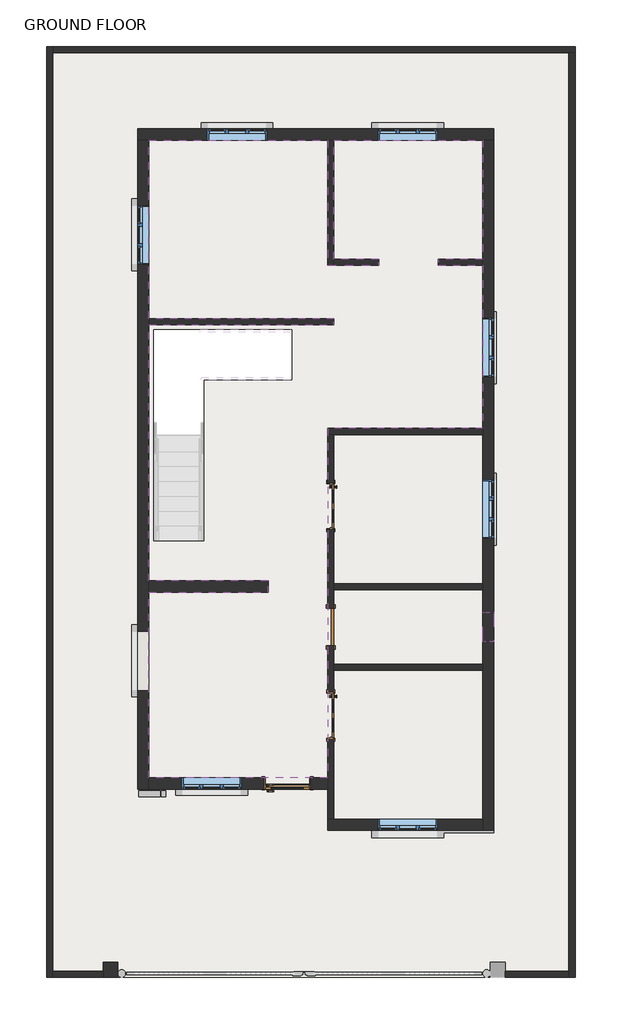
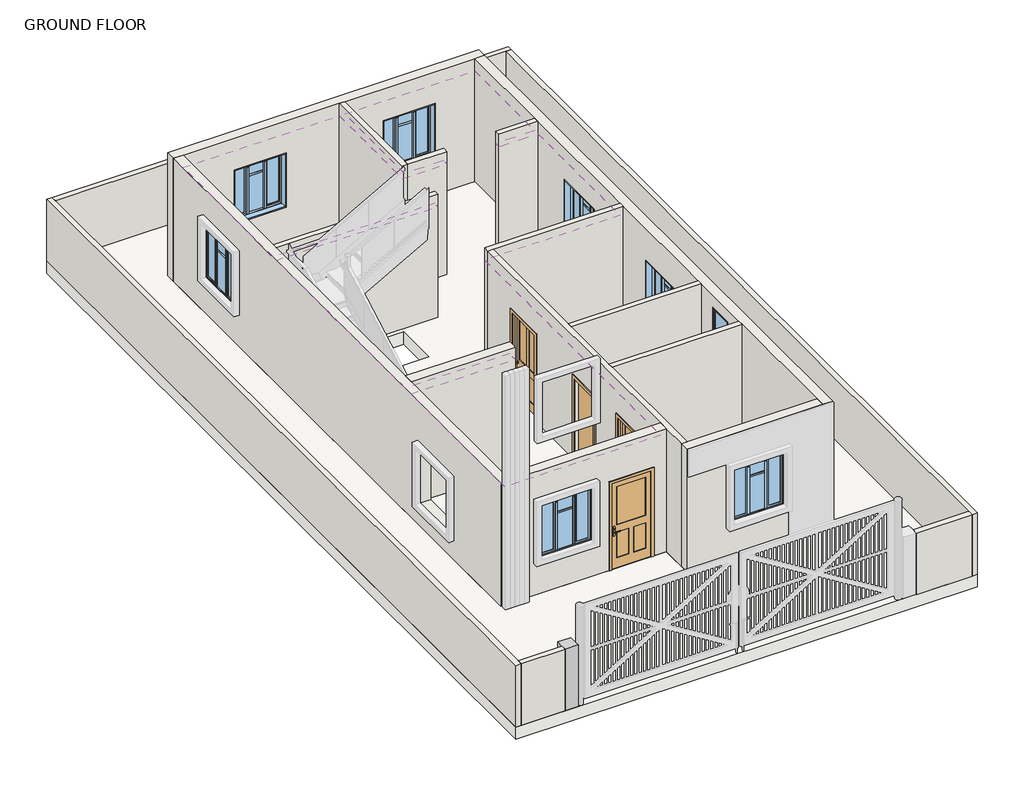
# One storey, part 1 of 4: 19 walls, 8 windows, 4 doors, 3 slabs, 1 column, 1 covering.
"""IFC4 building model written with IfcOpenShell, lengths in millimetres."""

from ifc_helpers import new_model, si_unit, frame, origin, origin_with_axes, place, context, project, spatial, polyline, outline, extrude, faceted_brep, transform, mapped, element, save
from components import door_16625766, door_interior_single_4_panel_wood_interior_common_door_3_x_7_68a706ac, door_e00f436c, window_80340324, window_casement_triple_middle_transom_windows_4_x4_273a115f

model = new_model("IFC4")

# Units and contexts
model_context = context("Model", 3, world=origin())
ifc_project = project(units=[si_unit("LENGTHUNIT", "METRE", prefix="MILLI")], contexts=[model_context])

# Site, building, storey
site = spatial("IfcSite", under=ifc_project)
building = spatial("IfcBuilding", under=site)
storey = spatial("IfcBuildingStorey", under=building, Name="GROUND FLOOR", Elevation=304.8)

# Column
placement = place(None, origin())
element("IfcColumn", 1, ObjectType="Rectangular Column : 1'X 1'", at=placement, inside=storey, context=model_context, shape_type="Brep", body=[
    faceted_brep([(-10104.8610805, -9269.5210084, 304.8), (-10104.8610805, -9574.3210084, 304.8), (-10409.6610805, -9574.3210084, 304.8), (-10409.6610805, -9447.3210084, 304.8), (-10409.6610805, -9269.5210084, 304.8), (-10104.8610805, -9269.5210084, 1828.8), (-10104.8610805, -9574.3210084, 1828.8), (-10409.6610805, -9574.3210084, 1828.8), (-10409.6610805, -9447.3210084, 1828.8), (-10409.6610805, -9269.5210084, 1828.8)], [[[0, 1, 2, 3, 4]], [[5, 6, 1, 0]], [[6, 7, 2, 1]], [[7, 8, 9, 4, 3, 2]], [[9, 5, 0, 4]], [[5, 9, 8, 7, 6]]]),
])

# Covering
element("IfcCovering", 2, ObjectType="2' x 4' ACT System", at=placement, inside=storey, context=model_context, shape_type="SweptSolid", body=[
    extrude(outline(polyline([(-9469.5482439, 3904.0172538), (-9469.5482439, 7561.6172538), (-5810.3607439, 7561.6172538), (-5810.3607439, 4996.2172538), (-4768.9607439, 4996.2172538), (-4768.9607439, 5123.2172538), (-5683.3607439, 5123.2172538), (-5683.3607439, 7561.6172538), (-2635.3607439, 7561.6172538), (-2635.3607439, 5123.2172538), (-3549.7607439, 5123.2172538), (-3549.7607439, 4996.2172538), (-2635.3607439, 4996.2172538), (-2635.3607439, 1659.1157342), (-5810.3607439, 1659.1157342), (-5810.3607439, -5493.9827462), (-9469.5482439, -5493.9827462), (-9469.5482439, -1691.1442658), (-7029.5607439, -1691.1442658), (-7029.5607439, -1462.5442658), (-9469.5482439, -1462.5442658), (-9469.5482439, 3777.0172538), (-5683.3607439, 3777.0172538), (-5683.3607439, 3904.0172538), (-9469.5482439, 3904.0172538)])), frame((0.0, 0.0, 3048.0), z_axis=(0.0, 0.0, 1.0), x_axis=(1.0, 0.0, 0.0)), (0.0, 0.0, 1.0), 57.15),
])

# Doors
door_shape = door_16625766(model_context)
element("IfcDoor", 3, ObjectType="36\" x 84\"", at=placement, inside=storey, context=model_context, shape_type="MappedRepresentation", body=[
    mapped(door_shape, transform((-6635.8607439, -5611.4577462, 304.8), x_axis=(-1.0, 0.0, 0.0), y_axis=(0.0, -1.0, 0.0), z_axis=(0.0, 0.0, 1.0))),
])
door_interior_single_4_panel_wood_interior_common_door_3_x_7_shape = door_interior_single_4_panel_wood_interior_common_door_3_x_7_68a706ac(model_context)
element("IfcDoor", 4, ObjectType="Door-Interior-Single-4_Panel-Wood : INTERIOR COMMON DOOR 3' X 7'", at=placement, inside=storey, context=model_context, shape_type="MappedRepresentation", body=[
    mapped(door_interior_single_4_panel_wood_interior_common_door_3_x_7_shape, transform((-5743.6857439, -4220.9842658, 304.8), x_axis=(0.0, -1.0, 0.0), y_axis=(1.0, 0.0, 0.0), z_axis=(0.0, 0.0, 1.0))),
])
element("IfcDoor", 5, ObjectType="Door-Interior-Single-4_Panel-Wood : INTERIOR COMMON DOOR 3' X 7'", at=placement, inside=storey, context=model_context, shape_type="MappedRepresentation", body=[
    mapped(door_interior_single_4_panel_wood_interior_common_door_3_x_7_shape, transform((-5743.6857439, 66.5357342, 304.8), x_axis=(0.0, -1.0, 0.0), y_axis=(1.0, 0.0, 0.0), z_axis=(0.0, 0.0, 1.0))),
])
door_2_shape = door_e00f436c(model_context)
element("IfcDoor", 6, ObjectType="Single-Flush : 30\" x 80\"", at=placement, inside=storey, context=model_context, shape_type="MappedRepresentation", body=[
    mapped(door_2_shape, transform((-5746.8607439, -2404.8842658, 304.8), x_axis=(0.0, 1.0, 0.0), y_axis=(-1.0, 0.0, 0.0), z_axis=(0.0, 0.0, 1.0))),
])

# Slabs
element("IfcSlab", 7, ObjectType="BATHROOM FLOORING 1'", at=placement, inside=storey, context=model_context, shape_type="SweptSolid", body=[
    extrude(outline(polyline([(-2635.3607439, -1642.8842658), (-2635.3607439, -3166.8842658), (-5683.3607439, -3166.8842658), (-5683.3607439, -1642.8842658), (-2635.3607439, -1642.8842658)])), origin_with_axes(), (0.0, 0.0, 1.0), 304.8),
])
element("IfcSlab", 8, ObjectType="FLOORING GROUND FLOOR 1'", at=placement, inside=storey, context=model_context, shape_type="SweptSolid", body=[
    extrude(outline(polyline([(-2406.7607439, 7790.2172538), (-2406.7607439, -6570.4842658), (-5810.3607439, -6570.4842658), (-5810.3607439, -5722.5827462), (-9698.1482439, -5722.5827462), (-9698.1482439, 7790.2172538), (-2406.7607439, 7790.2172538)]), holes=[polyline([(-2635.3607439, -1642.8842658), (-5683.3607439, -1642.8842658), (-5683.3607439, -3166.8842658), (-2635.3607439, -3166.8842658), (-2635.3607439, -1642.8842658)]), polyline([(-9367.9482439, 3675.4172538), (-9367.9482439, -642.5827462), (-8350.3607439, -642.5827462), (-8350.3607439, 2659.4172538), (-6542.1982439, 2659.4172538), (-6542.1982439, 3675.4172538), (-9367.9482439, 3675.4172538)])]), origin_with_axes(), (0.0, 0.0, 1.0), 304.8),
])
element("IfcSlab", 9, ObjectType="VERANDA FLOORING 1'", at=placement, inside=storey, context=model_context, shape_type="SweptSolid", body=[
    extrude(outline(polyline([(-744.9610805, 9475.6789916), (-744.9610805, -9574.3210084), (-11565.3610805, -9574.3210084), (-11565.3610805, 9475.6789916), (-744.9610805, 9475.6789916)]), holes=[polyline([(-2406.7607439, 7790.2172538), (-9698.1482439, 7790.2172538), (-9698.1482439, -5722.5827462), (-5810.3607439, -5722.5827462), (-5810.3607439, -6570.4842658), (-2406.7607439, -6570.4842658), (-2406.7607439, 7790.2172538)])]), origin_with_axes(), (0.0, 0.0, 1.0), 304.8),
])

# Walls
element("IfcWall", 10, ObjectType="INNER WALL 5\"", at=placement, inside=storey, context=model_context, shape_type="SweptSolid", body=[
    extrude(outline(polyline([(-5683.3607439, 3777.0172538), (-9469.5482439, 3777.0172538), (-9469.5482439, 3904.0172538), (-5683.3607439, 3904.0172538), (-5683.3607439, 3777.0172538)])), frame((0.0, 0.0, 304.8), z_axis=(0.0, 0.0, 1.0), x_axis=(1.0, 0.0, 0.0)), (0.0, 0.0, 1.0), 3048.0),
])
element("IfcWall", 11, ObjectType="INNER WALL 5\"", at=placement, inside=storey, context=model_context, shape_type="Brep", body=[
    faceted_brep([(-2635.3607439, 1659.1157342, 304.8), (-5810.3607439, 1659.1157342, 304.8), (-5810.3607439, 1659.1157342, 3352.8), (-2635.3607439, 1659.1157342, 3352.8), (-2635.3607439, 1532.1157342, 304.8), (-2635.3607439, 1532.1157342, 3352.8), (-5683.3607439, 1532.1157342, 3352.8), (-5810.3607439, 1532.1157342, 3352.8), (-5810.3607439, 1532.1157342, 304.8), (-5683.3607439, 1532.1157342, 304.8)], [[[0, 1, 2, 3]], [[4, 5, 6, 7, 8, 9]], [[1, 0, 4, 9, 8]], [[3, 2, 7, 6, 5]], [[0, 3, 5, 4]], [[2, 1, 8, 7]]]),
])
element("IfcWall", 12, ObjectType="INNER WALL 5\"", at=placement, inside=storey, context=model_context, shape_type="Brep", body=[
    faceted_brep([(-5810.3607439, -416.0642658, 304.8), (-5810.3607439, -2023.8842658, 304.8), (-5810.3607439, -2023.8842658, 2336.8), (-5810.3607439, -2785.8842658, 2336.8), (-5810.3607439, -2785.8842658, 304.8), (-5810.3607439, -3738.3842658, 304.8), (-5810.3607439, -3738.3842658, 2463.8), (-5810.3607439, -4703.5842658, 2463.8), (-5810.3607439, -4703.5842658, 304.8), (-5810.3607439, -5493.9827462, 304.8), (-5810.3607439, -5722.5827462, 304.8), (-5810.3607439, -6341.8842658, 304.8), (-5810.3607439, -6341.8842658, 3352.8), (-5810.3607439, -5722.5827462, 3352.8), (-5810.3607439, -5493.9827462, 3352.8), (-5810.3607439, 1532.1157342, 3352.8), (-5810.3607439, 1532.1157342, 304.8), (-5810.3607439, 549.1357342, 304.8), (-5810.3607439, 549.1357342, 2463.8), (-5810.3607439, -416.0642658, 2463.8), (-5683.3607439, -2023.8842658, 2336.8), (-5683.3607439, -2023.8842658, 304.8), (-5683.3607439, -1642.8842658, 304.8), (-5683.3607439, -1515.8842658, 304.8), (-5683.3607439, -416.0642658, 304.8), (-5683.3607439, -416.0642658, 2463.8), (-5683.3607439, 549.1357342, 2463.8), (-5683.3607439, 549.1357342, 304.8), (-5683.3607439, 1532.1157342, 304.8), (-5683.3607439, 1532.1157342, 3352.8), (-5683.3607439, -1515.8842658, 3352.8), (-5683.3607439, -1642.8842658, 3352.8), (-5683.3607439, -3166.8842658, 3352.8), (-5683.3607439, -3293.8842658, 3352.8), (-5683.3607439, -6341.8842658, 3352.8), (-5683.3607439, -6341.8842658, 304.8), (-5683.3607439, -4703.5842658, 304.8), (-5683.3607439, -4703.5842658, 2463.8), (-5683.3607439, -3738.3842658, 2463.8), (-5683.3607439, -3738.3842658, 304.8), (-5683.3607439, -3293.8842658, 304.8), (-5683.3607439, -3166.8842658, 304.8), (-5683.3607439, -2785.8842658, 304.8), (-5683.3607439, -2785.8842658, 2336.8)], [[[0, 1, 2, 3, 4, 5, 6, 7, 8, 9, 10, 11, 12, 13, 14, 15, 16, 17, 18, 19]], [[20, 21, 22, 23, 24, 25, 26, 27, 28, 29, 30, 31, 32, 33, 34, 35, 36, 37, 38, 39, 40, 41, 42, 43]], [[16, 28, 27, 17]], [[35, 11, 10, 9, 8, 36]], [[42, 41, 40, 39, 5, 4]], [[24, 23, 22, 21, 1, 0]], [[15, 14, 13, 12, 34, 33, 32, 31, 30, 29]], [[16, 15, 29, 28]], [[12, 11, 35, 34]], [[7, 37, 36, 8]], [[37, 7, 6, 38]], [[38, 6, 5, 39]], [[19, 25, 24, 0]], [[25, 19, 18, 26]], [[26, 18, 17, 27]], [[2, 1, 21, 20]], [[3, 2, 20, 43]], [[4, 3, 43, 42]]]),
])
element("IfcWall", 13, ObjectType="INNER WALL 5\"", at=placement, inside=storey, context=model_context, shape_type="SweptSolid", body=[
    extrude(outline(polyline([(-2635.3607439, -3293.8842658), (-5683.3607439, -3293.8842658), (-5683.3607439, -3166.8842658), (-2635.3607439, -3166.8842658), (-2635.3607439, -3293.8842658)])), frame((0.0, 0.0, 304.8), z_axis=(0.0, 0.0, 1.0), x_axis=(1.0, 0.0, 0.0)), (0.0, 0.0, 1.0), 3048.0),
])
element("IfcWall", 14, ObjectType="INNER WALL 5\"", at=placement, inside=storey, context=model_context, shape_type="SweptSolid", body=[
    extrude(outline(polyline([(-2635.3607439, -1642.8842658), (-5683.3607439, -1642.8842658), (-5683.3607439, -1515.8842658), (-2635.3607439, -1515.8842658), (-2635.3607439, -1642.8842658)])), frame((0.0, 0.0, 304.8), z_axis=(0.0, 0.0, 1.0), x_axis=(1.0, 0.0, 0.0)), (0.0, 0.0, 1.0), 3048.0),
])
element("IfcWall", 15, ObjectType="INNER WALL 5\"", at=placement, inside=storey, context=model_context, shape_type="Brep", body=[
    faceted_brep([(-5810.3607439, 7561.6172538, 304.8), (-5810.3607439, 4996.2172538, 304.8), (-5810.3607439, 4996.2172538, 3352.8), (-5810.3607439, 7561.6172538, 3352.8), (-5683.3607439, 7561.6172538, 304.8), (-5683.3607439, 7561.6172538, 3352.8), (-5683.3607439, 5123.2172538, 3352.8), (-5683.3607439, 4996.2172538, 3352.8), (-5683.3607439, 4996.2172538, 304.8), (-5683.3607439, 5123.2172538, 304.8)], [[[0, 1, 2, 3]], [[4, 5, 6, 7, 8, 9]], [[1, 0, 4, 9, 8]], [[3, 2, 7, 6, 5]], [[0, 3, 5, 4]], [[2, 1, 8, 7]]]),
])
element("IfcWall", 16, ObjectType="INNER WALL 5\"", at=placement, inside=storey, context=model_context, shape_type="SweptSolid", body=[
    extrude(outline(polyline([(-4768.9607439, 4996.2172538), (-5683.3607439, 4996.2172538), (-5683.3607439, 5123.2172538), (-4768.9607439, 5123.2172538), (-4768.9607439, 4996.2172538)])), frame((0.0, 0.0, 304.8), z_axis=(0.0, 0.0, 1.0), x_axis=(1.0, 0.0, 0.0)), (0.0, 0.0, 1.0), 3048.0),
])
element("IfcWall", 17, ObjectType="INNER WALL 5\"", at=placement, inside=storey, context=model_context, shape_type="SweptSolid", body=[
    extrude(outline(polyline([(-2635.3607439, 4996.2172538), (-3549.7607439, 4996.2172538), (-3549.7607439, 5123.2172538), (-2635.3607439, 5123.2172538), (-2635.3607439, 4996.2172538)])), frame((0.0, 0.0, 304.8), z_axis=(0.0, 0.0, 1.0), x_axis=(1.0, 0.0, 0.0)), (0.0, 0.0, 1.0), 3048.0),
])
element("IfcWall", 18, ObjectType="INNER WALL 5\"", at=placement, inside=storey, context=model_context, shape_type="Brep", body=[
    faceted_brep([(-11565.3610805, 9475.6789916, 304.8), (-11565.3610805, -9574.3210084, 304.8), (-11565.3610805, -9574.3210084, 1828.8), (-11565.3610805, 9475.6789916, 1828.8), (-11438.3610805, 9475.6789916, 304.8), (-11438.3610805, 9475.6789916, 1828.8), (-11438.3610805, 9348.6789916, 1828.8), (-11438.3610805, -9447.3210084, 1828.8), (-11438.3610805, -9574.3210084, 1828.8), (-11438.3610805, -9574.3210084, 304.8), (-11438.3610805, -9447.3210084, 304.8), (-11438.3610805, 9348.6789916, 304.8)], [[[0, 1, 2, 3]], [[4, 5, 6, 7, 8, 9, 10, 11]], [[1, 0, 4, 11, 10, 9]], [[3, 2, 8, 7, 6, 5]], [[0, 3, 5, 4]], [[2, 1, 9, 8]]]),
])
element("IfcWall", 19, ObjectType="INNER WALL 5\"", at=placement, inside=storey, context=model_context, shape_type="Brep", body=[
    faceted_brep([(-11438.3610805, 9348.6789916, 304.8), (-871.9610805, 9348.6789916, 304.8), (-744.9610805, 9348.6789916, 304.8), (-744.9610805, 9348.6789916, 1828.8), (-871.9610805, 9348.6789916, 1828.8), (-11438.3610805, 9348.6789916, 1828.8), (-11438.3610805, 9475.6789916, 304.8), (-11438.3610805, 9475.6789916, 1828.8), (-744.9610805, 9475.6789916, 1828.8), (-744.9610805, 9475.6789916, 304.8)], [[[0, 1, 2, 3, 4, 5]], [[6, 7, 8, 9]], [[2, 1, 0, 6, 9]], [[5, 4, 3, 8, 7]], [[0, 5, 7, 6]], [[3, 2, 9, 8]]]),
])
element("IfcWall", 20, ObjectType="INNER WALL 5\"", at=placement, inside=storey, context=model_context, shape_type="Brep", body=[
    faceted_brep([(-871.9610805, 9348.6789916, 304.8), (-871.9610805, -9447.3210084, 304.8), (-871.9610805, -9574.3210084, 304.8), (-871.9610805, -9574.3210084, 1828.8), (-871.9610805, -9447.3210084, 1828.8), (-871.9610805, 9348.6789916, 1828.8), (-744.9610805, 9348.6789916, 304.8), (-744.9610805, 9348.6789916, 1828.8), (-744.9610805, -9574.3210084, 1828.8), (-744.9610805, -9574.3210084, 304.8)], [[[0, 1, 2, 3, 4, 5]], [[6, 7, 8, 9]], [[2, 1, 0, 6, 9]], [[5, 4, 3, 8, 7]], [[0, 5, 7, 6]], [[3, 2, 9, 8]]]),
])
element("IfcWall", 21, ObjectType="INNER WALL 5\"", at=placement, inside=storey, context=model_context, shape_type="SweptSolid", body=[
    extrude(outline(polyline([(-2180.0610805, -9447.3210084), (-871.9610805, -9447.3210084), (-871.9610805, -9574.3210084), (-2180.0610805, -9574.3210084), (-2180.0610805, -9447.3210084)])), frame((0.0, 0.0, 304.8), z_axis=(0.0, 0.0, 1.0), x_axis=(1.0, 0.0, 0.0)), (0.0, 0.0, 1.0), 1524.0),
])
element("IfcWall", 22, ObjectType="INNER WALL 5\"", at=placement, inside=storey, context=model_context, shape_type="SweptSolid", body=[
    extrude(outline(polyline([(-10409.6610805, -9574.3210084), (-11438.3610805, -9574.3210084), (-11438.3610805, -9447.3210084), (-10409.6610805, -9447.3210084), (-10409.6610805, -9574.3210084)])), frame((0.0, 0.0, 304.8), z_axis=(0.0, 0.0, 1.0), x_axis=(1.0, 0.0, 0.0)), (0.0, 0.0, 1.0), 1524.0),
])
element("IfcWall", 23, ObjectType="WALL 9\"", at=placement, inside=storey, context=model_context, shape_type="Brep", body=[
    faceted_brep([(-9698.1482439, 7561.6172538, 304.8), (-9469.5482439, 7561.6172538, 304.8), (-5810.3607439, 7561.6172538, 304.8), (-5683.3607439, 7561.6172538, 304.8), (-2635.3607439, 7561.6172538, 304.8), (-2406.7607439, 7561.6172538, 304.8), (-2406.7607439, 7561.6172538, 3352.8), (-2635.3607439, 7561.6172538, 3352.8), (-5683.3607439, 7561.6172538, 3352.8), (-5810.3607439, 7561.6172538, 3352.8), (-9469.5482439, 7561.6172538, 3352.8), (-9698.1482439, 7561.6172538, 3352.8), (-7055.7544939, 7561.6172538, 2565.4), (-7055.7544939, 7561.6172538, 1219.2), (-8274.9544939, 7561.6172538, 1219.2), (-8274.9544939, 7561.6172538, 2565.4), (-3562.4607439, 7561.6172538, 2565.4), (-3562.4607439, 7561.6172538, 1219.2), (-4781.6607439, 7561.6172538, 1219.2), (-4781.6607439, 7561.6172538, 2565.4), (-9698.1482439, 7790.2172538, 304.8), (-9698.1482439, 7790.2172538, 3352.8), (-2406.7607439, 7790.2172538, 3352.8), (-2406.7607439, 7790.2172538, 304.8), (-7055.7544939, 7790.2172538, 2565.4), (-8274.9544939, 7790.2172538, 2565.4), (-8274.9544939, 7790.2172538, 1219.2), (-7055.7544939, 7790.2172538, 1219.2), (-3562.4607439, 7790.2172538, 2565.4), (-4781.6607439, 7790.2172538, 2565.4), (-4781.6607439, 7790.2172538, 1219.2), (-3562.4607439, 7790.2172538, 1219.2)], [[[0, 1, 2, 3, 4, 5, 6, 7, 8, 9, 10, 11], [12, 13, 14, 15], [16, 17, 18, 19]], [[20, 21, 22, 23], [24, 25, 26, 27], [28, 29, 30, 31]], [[5, 4, 3, 2, 1, 0, 20, 23]], [[11, 10, 9, 8, 7, 6, 22, 21]], [[6, 5, 23, 22]], [[0, 11, 21, 20]], [[13, 12, 24, 27]], [[14, 13, 27, 26]], [[15, 14, 26, 25]], [[12, 15, 25, 24]], [[17, 16, 28, 31]], [[18, 17, 31, 30]], [[19, 18, 30, 29]], [[16, 19, 29, 28]]]),
])
element("IfcWall", 24, ObjectType="WALL 9\"", at=placement, inside=storey, context=model_context, shape_type="Brep", body=[
    faceted_brep([(-2635.3607439, 7561.6172538, 304.8), (-2635.3607439, 5123.2172538, 304.8), (-2635.3607439, 4996.2172538, 304.8), (-2635.3607439, 1659.1157342, 304.8), (-2635.3607439, 1532.1157342, 304.8), (-2635.3607439, -1515.8842658, 304.8), (-2635.3607439, -1642.8842658, 304.8), (-2635.3607439, -3166.8842658, 304.8), (-2635.3607439, -3293.8842658, 304.8), (-2635.3607439, -6341.8842658, 304.8), (-2635.3607439, -6570.4842658, 304.8), (-2635.3607439, -6570.4842658, 3352.8), (-2635.3607439, -6341.8842658, 3352.8), (-2635.3607439, -3293.8842658, 3352.8), (-2635.3607439, -3166.8842658, 3352.8), (-2635.3607439, -1642.8842658, 3352.8), (-2635.3607439, -1515.8842658, 3352.8), (-2635.3607439, 1532.1157342, 3352.8), (-2635.3607439, 1659.1157342, 3352.8), (-2635.3607439, 4996.2172538, 3352.8), (-2635.3607439, 5123.2172538, 3352.8), (-2635.3607439, 7561.6172538, 3352.8), (-2635.3607439, 2705.366494, 2565.4), (-2635.3607439, 2705.366494, 1219.2), (-2635.3607439, 3924.566494, 1219.2), (-2635.3607439, 3924.566494, 2565.4), (-2635.3607439, -601.4842658, 2565.4), (-2635.3607439, -601.4842658, 1219.2), (-2635.3607439, 617.7157342, 1219.2), (-2635.3607439, 617.7157342, 2565.4), (-2635.3607439, -2100.0842658, 3048.0), (-2635.3607439, -2709.6842658, 3048.0), (-2635.3607439, -2709.6842658, 2438.4), (-2635.3607439, -2100.0842658, 2438.4), (-2406.7607439, 7561.6172538, 304.8), (-2406.7607439, 7561.6172538, 3352.8), (-2406.7607439, -6570.4842658, 3352.8), (-2406.7607439, -6570.4842658, 304.8), (-2406.7607439, 2705.366494, 2565.4), (-2406.7607439, 3924.566494, 2565.4), (-2406.7607439, 3924.566494, 1219.2), (-2406.7607439, 2705.366494, 1219.2), (-2406.7607439, -601.4842658, 2565.4), (-2406.7607439, 617.7157342, 2565.4), (-2406.7607439, 617.7157342, 1219.2), (-2406.7607439, -601.4842658, 1219.2), (-2406.7607439, -2100.0842658, 3048.0), (-2406.7607439, -2100.0842658, 2438.4), (-2406.7607439, -2709.6842658, 2438.4), (-2406.7607439, -2709.6842658, 3048.0)], [[[0, 1, 2, 3, 4, 5, 6, 7, 8, 9, 10, 11, 12, 13, 14, 15, 16, 17, 18, 19, 20, 21], [22, 23, 24, 25], [26, 27, 28, 29], [30, 31, 32, 33]], [[34, 35, 36, 37], [38, 39, 40, 41], [42, 43, 44, 45], [46, 47, 48, 49]], [[10, 9, 8, 7, 6, 5, 4, 3, 2, 1, 0, 34, 37]], [[21, 20, 19, 18, 17, 16, 15, 14, 13, 12, 11, 36, 35]], [[0, 21, 35, 34]], [[11, 10, 37, 36]], [[23, 22, 38, 41]], [[24, 23, 41, 40]], [[25, 24, 40, 39]], [[22, 25, 39, 38]], [[27, 26, 42, 45]], [[28, 27, 45, 44]], [[29, 28, 44, 43]], [[26, 29, 43, 42]], [[47, 46, 30, 33]], [[48, 47, 33, 32]], [[49, 48, 32, 31]], [[46, 49, 31, 30]]]),
])
element("IfcWall", 25, ObjectType="WALL 9\"", at=placement, inside=storey, context=model_context, shape_type="Brep", body=[
    faceted_brep([(-2635.3607439, -6341.8842658, 304.8), (-5683.3607439, -6341.8842658, 304.8), (-5810.3607439, -6341.8842658, 304.8), (-5810.3607439, -6341.8842658, 3352.8), (-5683.3607439, -6341.8842658, 3352.8), (-2635.3607439, -6341.8842658, 3352.8), (-4781.6607439, -6341.8842658, 2565.4), (-4781.6607439, -6341.8842658, 1219.2), (-3562.4607439, -6341.8842658, 1219.2), (-3562.4607439, -6341.8842658, 2565.4), (-2635.3607439, -6570.4842658, 304.8), (-2635.3607439, -6570.4842658, 3352.8), (-5810.3607439, -6570.4842658, 3352.8), (-5810.3607439, -6570.4842658, 304.8), (-4781.6607439, -6570.4842658, 2565.4), (-3562.4607439, -6570.4842658, 2565.4), (-3562.4607439, -6570.4842658, 1219.2), (-4781.6607439, -6570.4842658, 1219.2)], [[[0, 1, 2, 3, 4, 5], [6, 7, 8, 9]], [[10, 11, 12, 13], [14, 15, 16, 17]], [[2, 1, 0, 10, 13]], [[5, 4, 3, 12, 11]], [[0, 5, 11, 10]], [[3, 2, 13, 12]], [[7, 6, 14, 17]], [[8, 7, 17, 16]], [[9, 8, 16, 15]], [[6, 9, 15, 14]]]),
])
element("IfcWall", 26, ObjectType="WALL 9\"", at=placement, inside=storey, context=model_context, shape_type="Brep", body=[
    faceted_brep([(-9698.1482439, 7561.6172538, 304.8), (-9698.1482439, -5722.5827462, 304.8), (-9698.1482439, -5722.5827462, 3352.8), (-9698.1482439, 7561.6172538, 3352.8), (-9698.1482439, 6228.1172538, 2565.4), (-9698.1482439, 5008.9172538, 2565.4), (-9698.1482439, 5008.9172538, 1219.2), (-9698.1482439, 6228.1172538, 1219.2), (-9698.1482439, -2491.2442658, 2260.6), (-9698.1482439, -3710.4442658, 2260.6), (-9698.1482439, -3710.4442658, 914.4), (-9698.1482439, -2491.2442658, 914.4), (-9469.5482439, 7561.6172538, 304.8), (-9469.5482439, 7561.6172538, 3352.8), (-9469.5482439, 3904.0172538, 3352.8), (-9469.5482439, 3777.0172538, 3352.8), (-9469.5482439, -1462.5442658, 3352.8), (-9469.5482439, -1691.1442658, 3352.8), (-9469.5482439, -5493.9827462, 3352.8), (-9469.5482439, -5722.5827462, 3352.8), (-9469.5482439, -5722.5827462, 304.8), (-9469.5482439, -5493.9827462, 304.8), (-9469.5482439, -1691.1442658, 304.8), (-9469.5482439, -1462.5442658, 304.8), (-9469.5482439, 3777.0172538, 304.8), (-9469.5482439, 3904.0172538, 304.8), (-9469.5482439, 6228.1172538, 2565.4), (-9469.5482439, 6228.1172538, 1219.2), (-9469.5482439, 5008.9172538, 1219.2), (-9469.5482439, 5008.9172538, 2565.4), (-9469.5482439, -2491.2442658, 2260.6), (-9469.5482439, -2491.2442658, 914.4), (-9469.5482439, -3710.4442658, 914.4), (-9469.5482439, -3710.4442658, 2260.6)], [[[0, 1, 2, 3], [4, 5, 6, 7], [8, 9, 10, 11]], [[12, 13, 14, 15, 16, 17, 18, 19, 20, 21, 22, 23, 24, 25], [26, 27, 28, 29], [30, 31, 32, 33]], [[1, 0, 12, 25, 24, 23, 22, 21, 20]], [[3, 2, 19, 18, 17, 16, 15, 14, 13]], [[0, 3, 13, 12]], [[2, 1, 20, 19]], [[27, 26, 4, 7]], [[28, 27, 7, 6]], [[29, 28, 6, 5]], [[26, 29, 5, 4]], [[31, 30, 8, 11]], [[32, 31, 11, 10]], [[33, 32, 10, 9]], [[30, 33, 9, 8]]]),
])
element("IfcWall", 27, ObjectType="WALL 9\"", at=placement, inside=storey, context=model_context, shape_type="SweptSolid", body=[
    extrude(outline(polyline([(3352.8, -5810.3607439), (3352.8, -9469.5482439), (304.8, -9469.5482439), (304.8, -7118.4607439), (2463.8, -7118.4607439), (2463.8, -6153.2607439), (304.8, -6153.2607439), (304.8, -5810.3607439), (3352.8, -5810.3607439)]), holes=[polyline([(2565.4, -8796.4482439), (2565.4, -7577.2482439), (1219.2, -7577.2482439), (1219.2, -8796.4482439), (2565.4, -8796.4482439)])]), frame((0.0, -5722.5827462, 0.0), z_axis=(0.0, 1.0, 0.0), x_axis=(0.0, 0.0, 1.0)), (0.0, 0.0, 1.0), 228.6),
])
element("IfcWall", 28, ObjectType="WALL 9\"", at=placement, inside=storey, context=model_context, shape_type="SweptSolid", body=[
    extrude(outline(polyline([(-7029.5607439, -1691.1442658), (-9469.5482439, -1691.1442658), (-9469.5482439, -1462.5442658), (-7029.5607439, -1462.5442658), (-7029.5607439, -1691.1442658)])), frame((0.0, 0.0, 304.8), z_axis=(0.0, 0.0, 1.0), x_axis=(1.0, 0.0, 0.0)), (0.0, 0.0, 1.0), 3048.0),
])

# Windows
window_shape = window_80340324(model_context)
element("IfcWindow", 29, ObjectType="Fixed : 24\" x 24\"", at=placement, inside=storey, context=model_context, shape_type="MappedRepresentation", body=[
    mapped(window_shape, transform((-2521.0607439, -2366.7842658, 1524.0), x_axis=(0.0, 1.0, 0.0), y_axis=(-1.0, 0.0, 0.0), z_axis=(0.0, 0.0, 1.0))),
])
window_casement_triple_middle_transom_windows_4_x4_shape = window_casement_triple_middle_transom_windows_4_x4_273a115f(model_context)
element("IfcWindow", 30, ObjectType="Window-Casement-Triple-Middle-Transom : WINDOWS 4'X4'", at=placement, inside=storey, context=model_context, shape_type="MappedRepresentation", body=[
    mapped(window_casement_triple_middle_transom_windows_4_x4_shape, transform((-7665.3544939, 7675.9172538, 304.8), x_axis=(1.0, 0.0, 0.0), y_axis=(0.0, 1.0, 0.0), z_axis=(0.0, 0.0, 1.0))),
])
element("IfcWindow", 31, ObjectType="Window-Casement-Triple-Middle-Transom : WINDOWS 4'X4'", at=placement, inside=storey, context=model_context, shape_type="MappedRepresentation", body=[
    mapped(window_casement_triple_middle_transom_windows_4_x4_shape, transform((-4172.0607439, 7675.9172538, 304.8), x_axis=(1.0, 0.0, 0.0), y_axis=(0.0, 1.0, 0.0), z_axis=(0.0, 0.0, 1.0))),
])
element("IfcWindow", 32, ObjectType="Window-Casement-Triple-Middle-Transom : WINDOWS 4'X4'", at=placement, inside=storey, context=model_context, shape_type="MappedRepresentation", body=[
    mapped(window_casement_triple_middle_transom_windows_4_x4_shape, transform((-2521.0607439, 3314.966494, 304.8), x_axis=(0.0, -1.0, 0.0), y_axis=(1.0, 0.0, 0.0), z_axis=(0.0, 0.0, 1.0))),
])
element("IfcWindow", 33, ObjectType="Window-Casement-Triple-Middle-Transom : WINDOWS 4'X4'", at=placement, inside=storey, context=model_context, shape_type="MappedRepresentation", body=[
    mapped(window_casement_triple_middle_transom_windows_4_x4_shape, transform((-2521.0607439, 8.1157342, 304.8), x_axis=(0.0, -1.0, 0.0), y_axis=(1.0, 0.0, 0.0), z_axis=(0.0, 0.0, 1.0))),
])
element("IfcWindow", 34, ObjectType="Window-Casement-Triple-Middle-Transom : WINDOWS 4'X4'", at=placement, inside=storey, context=model_context, shape_type="MappedRepresentation", body=[
    mapped(window_casement_triple_middle_transom_windows_4_x4_shape, transform((-4172.0607439, -6456.1842658, 304.8), x_axis=(-1.0, 0.0, 0.0), y_axis=(0.0, -1.0, 0.0), z_axis=(0.0, 0.0, 1.0))),
])
element("IfcWindow", 35, ObjectType="Window-Casement-Triple-Middle-Transom : WINDOWS 4'X4'", at=placement, inside=storey, context=model_context, shape_type="MappedRepresentation", body=[
    mapped(window_casement_triple_middle_transom_windows_4_x4_shape, transform((-8186.8482439, -5608.2827462, 304.8), x_axis=(-1.0, 0.0, 0.0), y_axis=(0.0, -1.0, 0.0), z_axis=(0.0, 0.0, 1.0))),
])
element("IfcWindow", 36, ObjectType="Window-Casement-Triple-Middle-Transom : WINDOWS 4'X4'", at=placement, inside=storey, context=model_context, shape_type="MappedRepresentation", body=[
    mapped(window_casement_triple_middle_transom_windows_4_x4_shape, transform((-9583.8482439, 5618.5172538, 304.8), x_axis=(0.0, 1.0, 0.0), y_axis=(-1.0, 0.0, 0.0), z_axis=(0.0, 0.0, 1.0))),
])

save(model, "model.ifc")

# Revit data of these elements
# Type "Rectangular Column : 1'X 1'"
#   Assembly Code = "B1010200"
#   Depth = 1' - 0"
#   Offset Base = 0' - 0"
#   Offset Top = 0' - 0"
#   Width = 1' - 0"
# Type "2' x 4' ACT System"
#   Assembly Code = "C3030210"
#   built-in parameter 1002203 = 1 (stored number, unit not read)
#   built-in parameter 1002202 = 1 (stored number, unit not read)
#   Layers, outside or top first: 0' - 1 5/8" "Default" (function 1); 0' - 0 5/8" "Acoustic Ceiling Tile 24 x 48" (function 5)
# Type "36\" x 84\""
#   Type Mark = "8"
#   Assembly Code = "B2030100"
#   Analytic Construction = "French door, wood frame with single glass"
#   Top Rail = 0' - 4 3/4"
#   Threshold Offset [instance default] = 0' - 0 1/2"
#   Thickness = 0' - 1 3/8"
#   Thermal Resistance (R) = 1.0696 (h·ft²·°F)/BTU
#   Swing Angle [instance default] = 90.00°
#   Stiles = 0' - 4 3/4"
#   Rough Width = 3' - 2"
#   Rough Height = 7' - 1"
#   Lock Rail = 0' - 7 1/8"
#   Height = 7' - 0"
#   Width = 3' - 0"
#   Heat Transfer Coefficient (U) = 0.9350 BTU/(h·ft²·°F)
#   Door Offset [instance default] = 0' - 0"
#   Bottom Rail = 0' - 9 1/2"
#   Threshold [instance default] = yes
#   Function = 1
#   Exterior Trim [instance default] = yes
#   Trim Material = Cherry
#   Threshold Material = Cherry
#   Panel Material = Cherry
#   Glazing = Glass
#   Frame Material = Cherry
#   Door Handle Material = Aluminum
#   Visual Light Transmittance = 0
#   Solar Heat Gain Coefficient = 0
#   Wall Closure = (empty or 0)
#   Construction Type = (empty or 0)
# Type "Door-Interior-Single-4_Panel-Wood : INTERIOR COMMON DOOR 3' X 7'"
#   Type Mark = "11"
#   Assembly Code = "C1020300"
#   Analytic Construction = "Wooden"
#   Top Rail = 0' - 4 11/16"
#   Thickness = 0' - 1 3/8"
#   Thermal Resistance (R) = 2.5876 (h·ft²·°F)/BTU
#   Swing Angle [instance default] = 90.00°
#   Stiles = 0' - 4 3/4"
#   Rough Width = 3' - 2"
#   Rough Height = 7' - 1"
#   Mullion = 0' - 4 1/2"
#   Lock Rail = 0' - 7 1/2"
#   Height = 7' - 0"
#   Width = 3' - 0"
#   Heat Transfer Coefficient (U) = 0.3865 BTU/(h·ft²·°F)
#   Bottom Rail = 0' - 9 1/8"
#   Trim Material = Cherry
#   Panel Material = Cherry
#   Frame Material = Cherry
#   Door Handle Material = Aluminum
#   Visual Light Transmittance = 0
#   Solar Heat Gain Coefficient = 0
#   Wall Closure = (empty or 0)
#   Function = (empty or 0)
# Type "Single-Flush : 30\" x 80\""
#   Type Mark = "5"
#   Construction Type Id = "MDOOR"
#   Assembly Code = "C1020"
#   Analytic Construction = "Metal"
#   Thickness = 0' - 2"
#   Heat Transfer Coefficient (U) = 0.651978 BTU/(h·ft²·°F)
#   Height = 6' - 8"
#   Trim Projection Ext = 0' - 1"
#   Trim Projection Int = 0' - 1"
#   Trim Width = 0' - 3"
#   Width = 2' - 6"
#   Define Thermal Properties by = 1
#   Define Thermal Properties by = 1
#   Door Material = Door - Panel
#   Frame Material = Door - Frame
#   Visual Light Transmittance = 0
#   Solar Heat Gain Coefficient = 0
#   Function = (empty or 0)
#   Wall Closure = (empty or 0)
# Type "BATHROOM FLOORING 1'"
#   Assembly Code = "B1010"
#   Function = 0
#   Layers, outside or top first: 1' - 0" "BATHROOM FLOORING" (function 1)
# Type "FLOORING GROUND FLOOR 1'"
#   Assembly Code = "B1010"
#   Function = 0
#   Layers, outside or top first: 1' - 0" "MARBLE FLOORING 1'" (function 1)
# Type "VERANDA FLOORING 1'"
#   Assembly Code = "B1010"
#   Function = 0
#   Layers, outside or top first: 1' - 0" "VERANDA FLOORING" (function 1)
# Type "INNER WALL 5\""
#   Assembly Code = "B2010"
# Type "WALL 9\""
#   Assembly Code = "B2010"
# Type "Fixed : 24\" x 24\""
#   Type Mark = "3"
#   Construction Type Id = "GSP4R"
#   Assembly Code = "B2020100"
#   Analytic Construction = "1/8 in Pilkington single glazing"
#   Visual Light Transmittance = 0.9
#   Solar Heat Gain Coefficient = 0.78
#   Heat Transfer Coefficient (U) = 0.6496 BTU/(h·ft²·°F)
#   Height = 2' - 0"
#   Default Sill Height = 3' - 0"
#   Width = 2' - 0"
#   Window Inset = 0' - 0 3/4"
#   Define Thermal Properties by = 1
#   Define Thermal Properties by = 1
#   Glass Pane Material = Glass
#   Sash Material = Sash
#   Wall Closure = (empty or 0)
# Type "Window-Casement-Triple-Middle-Transom : WINDOWS 4'X4'"
#   Type Mark = "21"
#   Fire Rating = "0.5h"
#   Assembly Code = "B2020100"
#   Analytic Construction = "Double glazing - domestic"
#   Window Width = 1' - 4"
#   Window Inset [instance default] = 0' - 0 5/8"
#   Wall Thickness [instance default] = 0' - 6"
#   Visual Light Transmittance = 0.81
#   Transom Height Ratio = 0.3
#   Thermal Resistance (R) = 1.8146 (h·ft²·°F)/BTU
#   Solar Heat Gain Coefficient = 0.76
#   Rough Width = 4' - 0 1/2"
#   Rough Height = 4' - 5 1/2"
#   Heat Transfer Coefficient (U) = 0.5511 BTU/(h·ft²·°F)
#   Height = 4' - 5"
#   Transom Height = 1' - 3.9"
#   Frame Gap 3 [instance default] = 0' - 1 83/128"
#   Frame Gap 2 [instance default] = 0' - 0 5/8"
#   Frame Gap 1 = 0' - 1 51/128"
#   Default Sill Height = 3' - 0"
#   Width = 4' - 0"
#   Frame Material = Metal - Aluminum
#   Glass Panel Material = Glass
#   Wall Closure = (empty or 0)
# Element 1 (IfcColumn, "Rectangular Column : 1'X 1'")
#   Phase Created = New Construction
# Element 2 (IfcCovering, "2' x 4' ACT System")
#   Height Offset From Level = 9' - 0"
#   Phase Created = New Construction
#   Materials on its faces: "Acoustic Ceiling Tile 24 x 48", "Default"
# Element 3 (IfcDoor, "36\" x 84\"")
#   Threshold Offset = 0' - 0 1/2"
#   Swing Angle = 90.00°
#   Door Offset = 0' - 0"
#   Threshold = yes
#   Exterior Trim = yes
#   Phase Created = New Construction
#   Materials on its faces: "Cherry", "Aluminum", "Glass"
# Elements 4, 5 (IfcDoor, "Door-Interior-Single-4_Panel-Wood : INTERIOR COMMON DOOR 3' X 7'")
#   Swing Angle = 90.00°
#   Phase Created = New Construction
#   Materials on its faces: "Cherry", "Aluminum"
# Element 6 (IfcDoor, "Single-Flush : 30\" x 80\"")
#   Phase Created = New Construction
#   Materials on its faces: "Door - Frame", "Door - Panel"
# Element 7 (IfcSlab, "BATHROOM FLOORING 1'")
#   Height Offset From Level = 0' - 0"
#   Phase Created = New Construction
#   Materials on its faces: "BATHROOM FLOORING"
# Element 8 (IfcSlab, "FLOORING GROUND FLOOR 1'")
#   Height Offset From Level = 0' - 0"
#   Phase Created = New Construction
#   Materials on its faces: "MARBLE FLOORING 1'"
# Element 9 (IfcSlab, "VERANDA FLOORING 1'")
#   Height Offset From Level = 0' - 0"
#   Phase Created = New Construction
#   Materials on its faces: "VERANDA FLOORING"
# Elements 10, 11, 12, 13, 14, 15, 16, 17 (IfcWall, "INNER WALL 5\"")
#   Top Offset = 0' - 0"
#   Base Offset = 0' - 0"
#   wall height = 10' - 0"
#   Phase Created = New Construction
#   Base Constraint = GROUND FLOOR
#   Top Constraint = Level 2
#   Materials on its faces: "SAGE GREEN"
# Elements 18, 19, 20, 21, 22 (IfcWall, "INNER WALL 5\"")
#   Top Offset = 0' - 0"
#   Base Offset = 0' - 0"
#   Unconnected Height = 5' - 0"
#   wall height = 5' - 0"
#   Phase Created = New Construction
#   Base Constraint = GROUND FLOOR
# Elements 23, 24, 25, 26, 27, 28 (IfcWall, "WALL 9\"")
#   Top Offset = 0' - 0"
#   Base Offset = 0' - 0"
#   wall height = 10' - 0"
#   Phase Created = New Construction
#   Base Constraint = GROUND FLOOR
#   Top Constraint = Level 2
#   Materials on its faces: "SAGE GREEN"
# Element 29 (IfcWindow, "Fixed : 24\" x 24\"")
#   Mark = "12"
#   Phase Created = New Construction
#   Materials on its faces: "Sash", "Glass"
# Element 30 (IfcWindow, "Window-Casement-Triple-Middle-Transom : WINDOWS 4'X4'")
#   Mark = "5"
#   Window Inset = 0' - 0 5/8"
#   Frame Gap 3 = 0' - 1 83/128"
#   Frame Gap 2 = 0' - 0 5/8"
#   Phase Created = New Construction
#   Materials on its faces: "Metal - Aluminum", "Glass"
# Element 31 (IfcWindow, "Window-Casement-Triple-Middle-Transom : WINDOWS 4'X4'")
#   Mark = "6"
#   Window Inset = 0' - 0 5/8"
#   Frame Gap 3 = 0' - 1 83/128"
#   Frame Gap 2 = 0' - 0 5/8"
#   Phase Created = New Construction
#   Materials on its faces: "Metal - Aluminum", "Glass"
# Element 32 (IfcWindow, "Window-Casement-Triple-Middle-Transom : WINDOWS 4'X4'")
#   Mark = "7"
#   Window Inset = 0' - 0 5/8"
#   Frame Gap 3 = 0' - 1 83/128"
#   Frame Gap 2 = 0' - 0 5/8"
#   Phase Created = New Construction
#   Materials on its faces: "Metal - Aluminum", "Glass"
# Element 33 (IfcWindow, "Window-Casement-Triple-Middle-Transom : WINDOWS 4'X4'")
#   Mark = "8"
#   Window Inset = 0' - 0 5/8"
#   Frame Gap 3 = 0' - 1 83/128"
#   Frame Gap 2 = 0' - 0 5/8"
#   Phase Created = New Construction
#   Materials on its faces: "Metal - Aluminum", "Glass"
# Element 34 (IfcWindow, "Window-Casement-Triple-Middle-Transom : WINDOWS 4'X4'")
#   Mark = "9"
#   Window Inset = 0' - 0 5/8"
#   Frame Gap 3 = 0' - 1 83/128"
#   Frame Gap 2 = 0' - 0 5/8"
#   Phase Created = New Construction
#   Materials on its faces: "Metal - Aluminum", "Glass"
# Element 35 (IfcWindow, "Window-Casement-Triple-Middle-Transom : WINDOWS 4'X4'")
#   Mark = "10"
#   Window Inset = 0' - 0 5/8"
#   Frame Gap 3 = 0' - 1 83/128"
#   Frame Gap 2 = 0' - 0 5/8"
#   Phase Created = New Construction
#   Materials on its faces: "Metal - Aluminum", "Glass"
# Element 36 (IfcWindow, "Window-Casement-Triple-Middle-Transom : WINDOWS 4'X4'")
#   Mark = "11"
#   Window Inset = 0' - 0 5/8"
#   Frame Gap 3 = 0' - 1 83/128"
#   Frame Gap 2 = 0' - 0 5/8"
#   Phase Created = New Construction
#   Materials on its faces: "Metal - Aluminum", "Glass"
# Materials
#   "Default": colour RGB 127 127 127, transparency 0, Cost = 0
#   "Acoustic Ceiling Tile 24 x 48": class "Generic", colour RGB 229 229 229, transparency 0, Description = "Acoustic Ceiling Tile 24 x 48", Cost = 0
#   "Cherry": class "Wood", colour RGB 226 177 128, transparency 0, Description = "Prunus Serotina", Cost = 0
#   "Glass": class "Glass", colour RGB 0 128 192, transparency 0.75, Description = "Soda Lime Glass", Cost = 0
#   "Aluminum": class "Metal", colour RGB 247 247 247, transparency 0, Description = "Aluminum 6061", Cost = 0
#   "Door - Panel": class "Wood", colour RGB 210 159 95, transparency 0, Cost = 0
#   "Door - Frame": colour RGB 118 70 51, transparency 0, Cost = 0
#   "BATHROOM FLOORING": class "Generic", colour RGB 120 120 120, transparency 0, Cost = 0
#   "MARBLE FLOORING 1'": class "Generic", colour RGB 120 120 120, transparency 0, Cost = 0
#   "VERANDA FLOORING": class "Generic", colour RGB 120 120 120, transparency 0, Cost = 0
#   "Sash": class "Wood", colour RGB 224 178 126, transparency 0, Cost = 0
#   "Metal - Aluminum": class "Metal", colour RGB 247 247 247, transparency 0, Cost = 0
#   "SAGE GREEN": class "Generic", colour RGB 120 120 120, transparency 0, Cost = 0
# Room at (-4133.961, -4843.284) mm, phase "New Construction", upper level "GROUND FLOOR", upper offset 10' - 0", lower offset 0' - 0"
#   Number = "1"
#   Name = "BEDROOM"
# Room at (-4133.961, 8.116) mm, phase "New Construction", upper level "GROUND FLOOR", upper offset 10' - 0", lower offset 0' - 0"
#   Number = "2"
#   Name = "STUDY ROOM"
# Room at (-4133.961, -2404.884) mm, phase "New Construction", upper level "GROUND FLOOR", upper offset 10' - 0", lower offset 0' - 0"
#   Number = "3"
#   Name = "TOILET"
# Room at (-7633.604, 5758.217) mm, phase "New Construction", upper level "GROUND FLOOR", upper offset 10' - 0", lower offset 0' - 0"
#   Number = "4"
#   Name = "LIVING ROOM"
# Room at (-4133.961, 6336.067) mm, phase "New Construction", upper level "GROUND FLOOR", upper offset 10' - 0", lower offset 0' - 0"
#   Number = "5"
#   Name = "KITCHEN"
# Room at (-7665.354, -3535.414) mm, phase "New Construction", upper level "GROUND FLOOR", upper offset 10' - 0", lower offset 0' - 0"
#   Number = "6"
#   Name = "FAMILY LOUNGE"
# Room at (-4102.211, 3327.666) mm, phase "New Construction", upper level "GROUND FLOOR", upper offset 10' - 0", lower offset 0' - 0"
#   Number = "7"
# Room at (-7633.604, 1131.836) mm, phase "New Construction", upper level "GROUND FLOOR", upper offset 10' - 0", lower offset 0' - 0"
#   Number = "8"
#   Name = "STAIRS"
